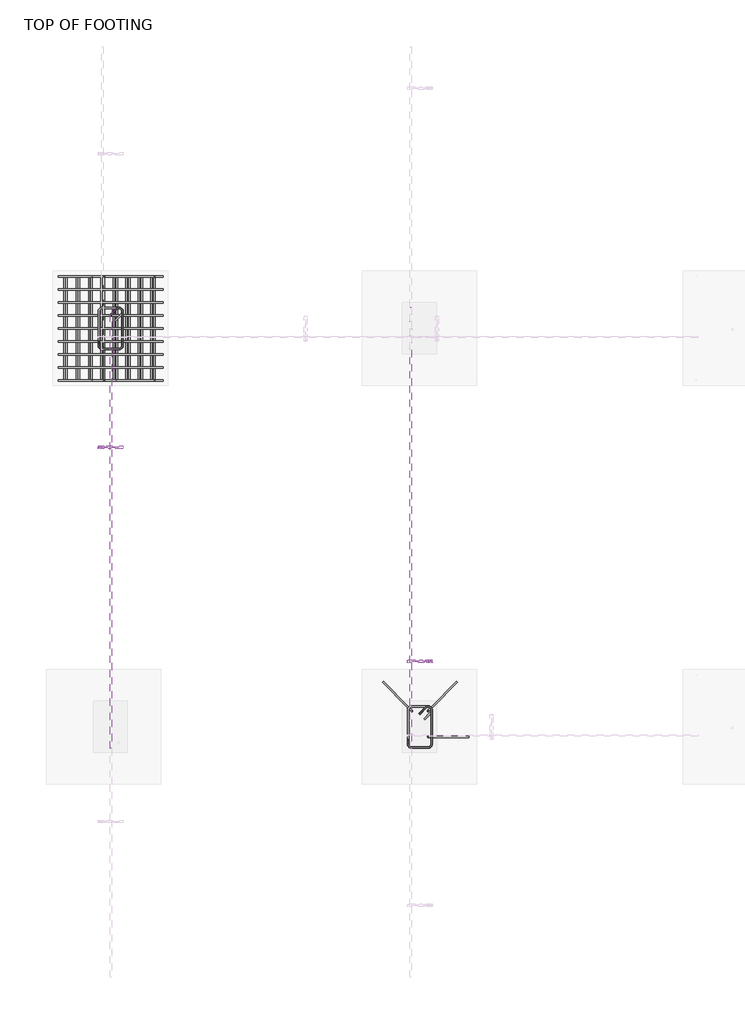
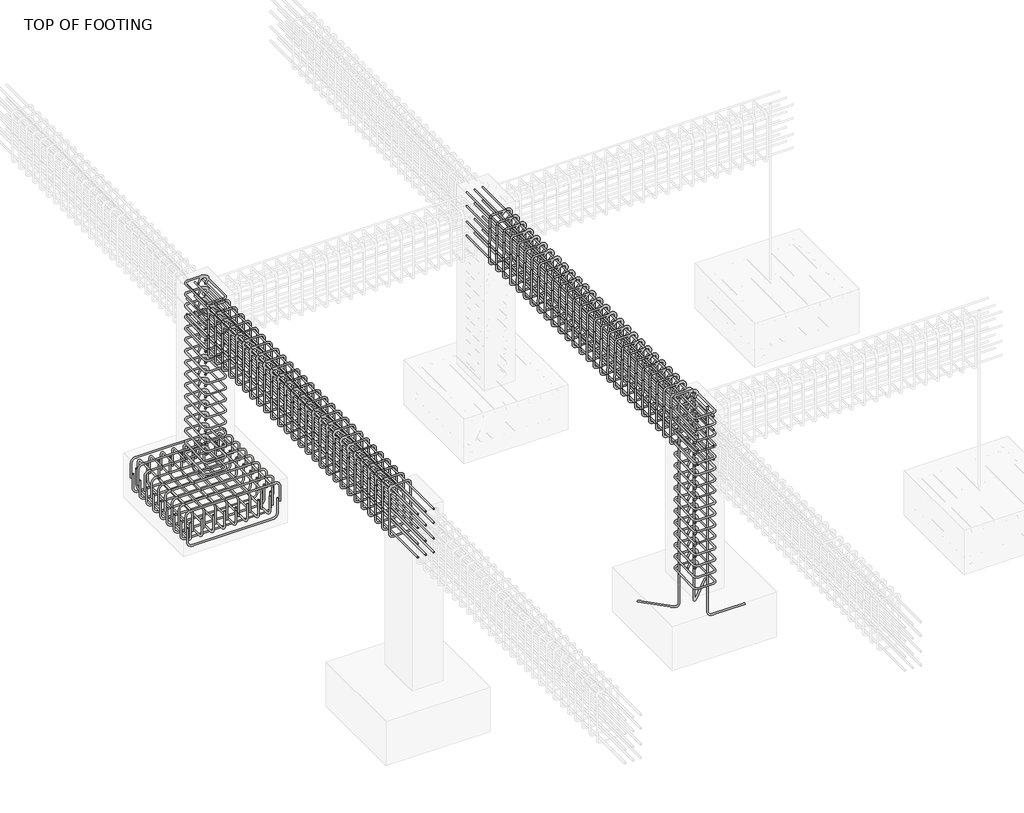
# One storey, part 6 of 14: 19 reinforcing bars.
"""IFC4 building model written with IfcOpenShell, lengths in millimetres."""

from ifc_helpers import new_model, si_unit, point, frame, origin, place, context, project, spatial, polyline, circle_curve, trimmed, segment, composite_curve, source, transform, mapped, element, save
from ifc_brep_helpers import swept_disk

model = new_model("IFC4")

# Units and contexts
model_context = context("Model", 3, world=origin())
ifc_project = project(units=[si_unit("LENGTHUNIT", "METRE", prefix="MILLI")], contexts=[model_context])

# Site, building, storey
site = spatial("IfcSite", under=ifc_project)
building = spatial("IfcBuilding", under=site)
storey = spatial("IfcBuildingStorey", under=building, Name="TOP OF FOOTING", Elevation=-1828.8)

# Reinforcing bars
placement = place(None, origin())
reinforcing_bar_shape = source(origin(), model_context, "Body", "SolidModel", [
    swept_disk(composite_curve([segment(polyline([(-3027.457813, 7055.1438575, -2035.6107622), (-3027.457813, 7055.1438575, -2182.9107622)]), True, "CONTINUOUS"), segment(trimmed(circle_curve(frame((-3073.807813, 7055.1438575, -2182.9107622), z_axis=(0.0, 1.0, 0.0), x_axis=(46.34999999999991, 0.0, 0.0)), 46.35), [point((-3027.457813, 7055.1438575, -2182.9107622))], [point((-3073.807813, 7055.1438575, -2229.2607622))], True, "CARTESIAN"), True, "CONTINUOUS"), segment(polyline([(-3073.807813, 7055.1438575, -2229.2607622), (-3846.4382016, 7055.1438575, -2229.2607622)]), True, "CONTINUOUS"), segment(trimmed(circle_curve(frame((-3846.4382016, 7055.1438575, -2182.9107622), z_axis=(0.0, 1.0, 0.0), x_axis=(0.0, 0.0, -46.34999999999991)), 46.35), [point((-3846.4382016, 7055.1438575, -2229.2607622))], [point((-3892.7882016, 7055.1438575, -2182.9107622))], True, "CARTESIAN"), True, "CONTINUOUS"), segment(polyline([(-3892.7882016, 7055.1438575, -2182.9107622), (-3892.7882016, 7055.1438575, -2035.6107622)]), True, "CONTINUOUS")], self_intersect=False), 6.35),
])
element("IfcReinforcingBar", 1, at=placement, inside=storey, context=model_context, shape_type="MappedRepresentation", body=[
    mapped(reinforcing_bar_shape, transform((0.0, 0.0, 0.0), x_axis=(1.0, 0.0, 0.0), y_axis=(0.0, 1.0, 0.0), z_axis=(0.0, 0.0, 1.0))),
    mapped(reinforcing_bar_shape, transform((0.0, -113.4125, 0.0), x_axis=(1.0, 0.0, 0.0), y_axis=(0.0, 1.0, 0.0), z_axis=(0.0, 0.0, 1.0))),
    mapped(reinforcing_bar_shape, transform((0.0, -226.825, 0.0), x_axis=(1.0, 0.0, 0.0), y_axis=(0.0, 1.0, 0.0), z_axis=(0.0, 0.0, 1.0))),
    mapped(reinforcing_bar_shape, transform((0.0, -340.2375, 0.0), x_axis=(1.0, 0.0, 0.0), y_axis=(0.0, 1.0, 0.0), z_axis=(0.0, 0.0, 1.0))),
    mapped(reinforcing_bar_shape, transform((0.0, -453.65, 0.0), x_axis=(1.0, 0.0, 0.0), y_axis=(0.0, 1.0, 0.0), z_axis=(0.0, 0.0, 1.0))),
    mapped(reinforcing_bar_shape, transform((0.0, -567.0625, 0.0), x_axis=(1.0, 0.0, 0.0), y_axis=(0.0, 1.0, 0.0), z_axis=(0.0, 0.0, 1.0))),
    mapped(reinforcing_bar_shape, transform((0.0, -680.475, 0.0), x_axis=(1.0, 0.0, 0.0), y_axis=(0.0, 1.0, 0.0), z_axis=(0.0, 0.0, 1.0))),
    mapped(reinforcing_bar_shape, transform((0.0, -793.8875, 0.0), x_axis=(1.0, 0.0, 0.0), y_axis=(0.0, 1.0, 0.0), z_axis=(0.0, 0.0, 1.0))),
    mapped(reinforcing_bar_shape, transform((0.0, -907.3, 0.0), x_axis=(1.0, 0.0, 0.0), y_axis=(0.0, 1.0, 0.0), z_axis=(0.0, 0.0, 1.0))),
])
reinforcing_bar_2_shape = source(origin(), model_context, "Body", "SolidModel", [
    swept_disk(composite_curve([segment(polyline([(-3911.0033787, 7055.1438575, -2068.991024), (-3911.0033787, 7055.1438575, -1921.691024)]), True, "CONTINUOUS"), segment(trimmed(circle_curve(frame((-3864.6533787, 7055.1438575, -1921.691024), z_axis=(0.0, 1.0, 0.0), x_axis=(-46.350000000000364, 0.0, 0.0)), 46.35), [point((-3911.0033787, 7055.1438575, -1921.691024))], [point((-3864.6533787, 7055.1438575, -1875.341024))], True, "CARTESIAN"), True, "CONTINUOUS"), segment(polyline([(-3864.6533787, 7055.1438575, -1875.341024), (-3050.0533787, 7055.1438575, -1875.341024)]), True, "CONTINUOUS"), segment(trimmed(circle_curve(frame((-3050.0533787, 7055.1438575, -1921.691024), z_axis=(0.0, 1.0, 0.0), x_axis=(0.0, 0.0, 46.34999999999991)), 46.35), [point((-3050.0533787, 7055.1438575, -1875.341024))], [point((-3003.7033787, 7055.1438575, -1921.691024))], True, "CARTESIAN"), True, "CONTINUOUS"), segment(polyline([(-3003.7033787, 7055.1438575, -1921.691024), (-3003.7033787, 7055.1438575, -2068.991024)]), True, "CONTINUOUS")], self_intersect=False), 6.35),
])
element("IfcReinforcingBar", 2, at=placement, inside=storey, context=model_context, shape_type="MappedRepresentation", body=[
    mapped(reinforcing_bar_2_shape, transform((0.0, 0.0, 0.0), x_axis=(1.0, 0.0, 0.0), y_axis=(0.0, 1.0, 0.0), z_axis=(0.0, 0.0, 1.0))),
    mapped(reinforcing_bar_2_shape, transform((0.0, -113.4125, 0.0), x_axis=(1.0, 0.0, 0.0), y_axis=(0.0, 1.0, 0.0), z_axis=(0.0, 0.0, 1.0))),
    mapped(reinforcing_bar_2_shape, transform((0.0, -226.825, 0.0), x_axis=(1.0, 0.0, 0.0), y_axis=(0.0, 1.0, 0.0), z_axis=(0.0, 0.0, 1.0))),
    mapped(reinforcing_bar_2_shape, transform((0.0, -340.2375, 0.0), x_axis=(1.0, 0.0, 0.0), y_axis=(0.0, 1.0, 0.0), z_axis=(0.0, 0.0, 1.0))),
    mapped(reinforcing_bar_2_shape, transform((0.0, -453.65, 0.0), x_axis=(1.0, 0.0, 0.0), y_axis=(0.0, 1.0, 0.0), z_axis=(0.0, 0.0, 1.0))),
    mapped(reinforcing_bar_2_shape, transform((0.0, -567.0625, 0.0), x_axis=(1.0, 0.0, 0.0), y_axis=(0.0, 1.0, 0.0), z_axis=(0.0, 0.0, 1.0))),
    mapped(reinforcing_bar_2_shape, transform((0.0, -680.475, 0.0), x_axis=(1.0, 0.0, 0.0), y_axis=(0.0, 1.0, 0.0), z_axis=(0.0, 0.0, 1.0))),
    mapped(reinforcing_bar_2_shape, transform((0.0, -793.8875, 0.0), x_axis=(1.0, 0.0, 0.0), y_axis=(0.0, 1.0, 0.0), z_axis=(0.0, 0.0, 1.0))),
    mapped(reinforcing_bar_2_shape, transform((0.0, -907.3, 0.0), x_axis=(1.0, 0.0, 0.0), y_axis=(0.0, 1.0, 0.0), z_axis=(0.0, 0.0, 1.0))),
])
reinforcing_bar_3_shape = source(origin(), model_context, "Body", "SolidModel", [
    swept_disk(composite_curve([segment(polyline([(-3073.4932847, 7055.1438575, -2085.4684936), (-3073.4932847, 7055.1438575, -1938.1684936)]), True, "CONTINUOUS"), segment(trimmed(circle_curve(frame((-3073.4932847, 7008.7938575, -1938.1684936), z_axis=(1.0, 0.0, 0.0), x_axis=(0.0, 46.350000000000364, 0.0)), 46.35), [point((-3073.4932847, 7055.1438575, -1938.1684936))], [point((-3073.4932847, 7008.7938575, -1891.8184936))], True, "CARTESIAN"), True, "CONTINUOUS"), segment(polyline([(-3073.4932847, 7008.7938575, -1891.8184936), (-3073.4932847, 6194.1938575, -1891.8184936)]), True, "CONTINUOUS"), segment(trimmed(circle_curve(frame((-3073.4932847, 6194.1938575, -1938.1684936), z_axis=(1.0, 0.0, 0.0), x_axis=(0.0, 0.0, 46.34999999999991)), 46.35), [point((-3073.4932847, 6194.1938575, -1891.8184936))], [point((-3073.4932847, 6147.8438575, -1938.1684936))], True, "CARTESIAN"), True, "CONTINUOUS"), segment(polyline([(-3073.4932847, 6147.8438575, -1938.1684936), (-3073.4932847, 6147.8438575, -2085.4684936)]), True, "CONTINUOUS")], self_intersect=False), 6.35),
])
element("IfcReinforcingBar", 3, at=placement, inside=storey, context=model_context, shape_type="MappedRepresentation", body=[
    mapped(reinforcing_bar_3_shape, transform((0.0, 0.0, 0.0), x_axis=(1.0, 0.0, 0.0), y_axis=(0.0, 1.0, 0.0), z_axis=(0.0, 0.0, 1.0))),
    mapped(reinforcing_bar_3_shape, transform((-110.0713853, 0.0, 0.0), x_axis=(1.0, 0.0, 0.0), y_axis=(0.0, 1.0, 0.0), z_axis=(0.0, 0.0, 1.0))),
    mapped(reinforcing_bar_3_shape, transform((-220.1427706, 0.0, 0.0), x_axis=(1.0, 0.0, 0.0), y_axis=(0.0, 1.0, 0.0), z_axis=(0.0, 0.0, 1.0))),
    mapped(reinforcing_bar_3_shape, transform((-330.2141558, 0.0, 0.0), x_axis=(1.0, 0.0, 0.0), y_axis=(0.0, 1.0, 0.0), z_axis=(0.0, 0.0, 1.0))),
    mapped(reinforcing_bar_3_shape, transform((-440.2855411, 0.0, 0.0), x_axis=(1.0, 0.0, 0.0), y_axis=(0.0, 1.0, 0.0), z_axis=(0.0, 0.0, 1.0))),
    mapped(reinforcing_bar_3_shape, transform((-550.3569264, 0.0, 0.0), x_axis=(1.0, 0.0, 0.0), y_axis=(0.0, 1.0, 0.0), z_axis=(0.0, 0.0, 1.0))),
    mapped(reinforcing_bar_3_shape, transform((-660.4283117, 0.0, 0.0), x_axis=(1.0, 0.0, 0.0), y_axis=(0.0, 1.0, 0.0), z_axis=(0.0, 0.0, 1.0))),
    mapped(reinforcing_bar_3_shape, transform((-770.4996969, 0.0, 0.0), x_axis=(1.0, 0.0, 0.0), y_axis=(0.0, 1.0, 0.0), z_axis=(0.0, 0.0, 1.0))),
])
reinforcing_bar_4_shape = source(origin(), model_context, "Body", "SolidModel", [
    swept_disk(composite_curve([segment(polyline([(-3862.3533787, 7055.1438575, -1990.15), (-3862.3533787, 7055.1438575, -2137.45)]), True, "CONTINUOUS"), segment(trimmed(circle_curve(frame((-3862.3533787, 7008.7938575, -2137.45), z_axis=(-1.0, 0.0, 0.0), x_axis=(0.0, 46.350000000000364, 0.0)), 46.35), [point((-3862.3533787, 7055.1438575, -2137.45))], [point((-3862.3533787, 7008.7938575, -2183.8))], True, "CARTESIAN"), True, "CONTINUOUS"), segment(polyline([(-3862.3533787, 7008.7938575, -2183.8), (-3862.3533787, 6194.1938575, -2183.8)]), True, "CONTINUOUS"), segment(trimmed(circle_curve(frame((-3862.3533787, 6194.1938575, -2137.45), z_axis=(-1.0, 0.0, 0.0), x_axis=(0.0, 0.0, -46.350000000000364)), 46.35), [point((-3862.3533787, 6194.1938575, -2183.8))], [point((-3862.3533787, 6147.8438575, -2137.45))], True, "CARTESIAN"), True, "CONTINUOUS"), segment(polyline([(-3862.3533787, 6147.8438575, -2137.45), (-3862.3533787, 6147.8438575, -1990.15)]), True, "CONTINUOUS")], self_intersect=False), 6.35),
])
element("IfcReinforcingBar", 4, at=placement, inside=storey, context=model_context, shape_type="MappedRepresentation", body=[
    mapped(reinforcing_bar_4_shape, transform((0.0, 0.0, 0.0), x_axis=(1.0, 0.0, 0.0), y_axis=(0.0, 1.0, 0.0), z_axis=(0.0, 0.0, 1.0))),
    mapped(reinforcing_bar_4_shape, transform((108.7810905, 0.0, 0.0), x_axis=(1.0, 0.0, 0.0), y_axis=(0.0, 1.0, 0.0), z_axis=(0.0, 0.0, 1.0))),
    mapped(reinforcing_bar_4_shape, transform((217.5621811, 0.0, 0.0), x_axis=(1.0, 0.0, 0.0), y_axis=(0.0, 1.0, 0.0), z_axis=(0.0, 0.0, 1.0))),
    mapped(reinforcing_bar_4_shape, transform((326.3432716, 0.0, 0.0), x_axis=(1.0, 0.0, 0.0), y_axis=(0.0, 1.0, 0.0), z_axis=(0.0, 0.0, 1.0))),
    mapped(reinforcing_bar_4_shape, transform((435.1243621, 0.0, 0.0), x_axis=(1.0, 0.0, 0.0), y_axis=(0.0, 1.0, 0.0), z_axis=(0.0, 0.0, 1.0))),
    mapped(reinforcing_bar_4_shape, transform((543.9054526, 0.0, 0.0), x_axis=(1.0, 0.0, 0.0), y_axis=(0.0, 1.0, 0.0), z_axis=(0.0, 0.0, 1.0))),
    mapped(reinforcing_bar_4_shape, transform((652.6865432, 0.0, 0.0), x_axis=(1.0, 0.0, 0.0), y_axis=(0.0, 1.0, 0.0), z_axis=(0.0, 0.0, 1.0))),
    mapped(reinforcing_bar_4_shape, transform((761.4676337, 0.0, 0.0), x_axis=(1.0, 0.0, 0.0), y_axis=(0.0, 1.0, 0.0), z_axis=(0.0, 0.0, 1.0))),
])
reinforcing_bar_5_shape = source(origin(), model_context, "Body", "SolidModel", [
    swept_disk(composite_curve([segment(polyline([(-3462.9647392, 6715.2180921, -46.35), (-3407.2211763, 6770.9616551, -46.35)]), True, "CONTINUOUS"), segment(trimmed(circle_curve(frame((-3385.0533787, 6748.7938575, -46.35), z_axis=(0.0, 0.0, -1.0), x_axis=(-22.167797600000085, 22.167797600000085, 0.0)), 31.35), [point((-3407.2211763, 6770.9616551, -46.35))], [point((-3353.7033787, 6748.7938575, -46.35))], True, "CARTESIAN"), True, "CONTINUOUS"), segment(polyline([(-3353.7033787, 6748.7938575, -46.35), (-3353.7033787, 6454.1938575, -46.35)]), True, "CONTINUOUS"), segment(trimmed(circle_curve(frame((-3385.0533787, 6454.1938575, -46.35), z_axis=(0.0, 0.0, -1.0), x_axis=(31.34999999999991, 0.0, 0.0)), 31.35), [point((-3353.7033787, 6454.1938575, -46.35))], [point((-3385.0533787, 6422.8438575, -46.35))], True, "CARTESIAN"), True, "CONTINUOUS"), segment(polyline([(-3385.0533787, 6422.8438575, -46.35), (-3529.6533787, 6422.8438575, -46.35)]), True, "CONTINUOUS"), segment(trimmed(circle_curve(frame((-3529.6533787, 6454.1740724, -45.2363875), z_axis=(0.0, 0.03552192833448213, -0.9993688971583016), x_axis=(0.0, -31.3302149000001, -1.1136125000000021)), 31.35), [point((-3529.6533787, 6422.8438575, -46.35))], [point((-3561.0033787, 6454.1740724, -45.2363875))], True, "CARTESIAN"), True, "CONTINUOUS"), segment(polyline([(-3561.0033787, 6454.1740724, -45.2363875), (-3561.0033787, 6748.8136426, -34.7636125)]), True, "CONTINUOUS"), segment(trimmed(circle_curve(frame((-3529.6533787, 6748.8136426, -34.7636125), z_axis=(0.0, 0.03552192833448213, -0.9993688971583016), x_axis=(-31.350000000000364, 0.0, 0.0)), 31.35), [point((-3561.0033787, 6748.8136426, -34.7636125))], [point((-3529.6533787, 6780.1438575, -33.65))], True, "CARTESIAN"), True, "CONTINUOUS"), segment(polyline([(-3529.6533787, 6780.1438575, -33.65), (-3385.0533787, 6780.1438575, -33.65)]), True, "CONTINUOUS"), segment(trimmed(circle_curve(frame((-3385.0533787, 6748.7938575, -33.65), z_axis=(0.0, 0.0, -1.0), x_axis=(0.0, 31.350000000000364, 0.0)), 31.35), [point((-3385.0533787, 6780.1438575, -33.65))], [point((-3362.8855811, 6726.6260599, -33.65))], True, "CARTESIAN"), True, "CONTINUOUS"), segment(polyline([(-3362.8855811, 6726.6260599, -33.65), (-3418.6291441, 6670.8824969, -33.65)]), True, "CONTINUOUS")], self_intersect=False), 6.35),
])
element("IfcReinforcingBar", 5, at=placement, inside=storey, context=model_context, shape_type="MappedRepresentation", body=[
    mapped(reinforcing_bar_5_shape, transform((0.0, 0.0, 0.0), x_axis=(1.0, 0.0, 0.0), y_axis=(0.0, 1.0, 0.0), z_axis=(0.0, 0.0, 1.0))),
    mapped(reinforcing_bar_5_shape, transform((0.0, 0.0, -115.74), x_axis=(1.0, 0.0, 0.0), y_axis=(0.0, 1.0, 0.0), z_axis=(0.0, 0.0, 1.0))),
    mapped(reinforcing_bar_5_shape, transform((0.0, 0.0, -231.48), x_axis=(1.0, 0.0, 0.0), y_axis=(0.0, 1.0, 0.0), z_axis=(0.0, 0.0, 1.0))),
    mapped(reinforcing_bar_5_shape, transform((0.0, 0.0, -347.22), x_axis=(1.0, 0.0, 0.0), y_axis=(0.0, 1.0, 0.0), z_axis=(0.0, 0.0, 1.0))),
    mapped(reinforcing_bar_5_shape, transform((0.0, 0.0, -462.96), x_axis=(1.0, 0.0, 0.0), y_axis=(0.0, 1.0, 0.0), z_axis=(0.0, 0.0, 1.0))),
    mapped(reinforcing_bar_5_shape, transform((0.0, 0.0, -578.7), x_axis=(1.0, 0.0, 0.0), y_axis=(0.0, 1.0, 0.0), z_axis=(0.0, 0.0, 1.0))),
    mapped(reinforcing_bar_5_shape, transform((0.0, 0.0, -694.44), x_axis=(1.0, 0.0, 0.0), y_axis=(0.0, 1.0, 0.0), z_axis=(0.0, 0.0, 1.0))),
    mapped(reinforcing_bar_5_shape, transform((0.0, 0.0, -810.18), x_axis=(1.0, 0.0, 0.0), y_axis=(0.0, 1.0, 0.0), z_axis=(0.0, 0.0, 1.0))),
    mapped(reinforcing_bar_5_shape, transform((0.0, 0.0, -925.92), x_axis=(1.0, 0.0, 0.0), y_axis=(0.0, 1.0, 0.0), z_axis=(0.0, 0.0, 1.0))),
    mapped(reinforcing_bar_5_shape, transform((0.0, 0.0, -1041.66), x_axis=(1.0, 0.0, 0.0), y_axis=(0.0, 1.0, 0.0), z_axis=(0.0, 0.0, 1.0))),
    mapped(reinforcing_bar_5_shape, transform((0.0, 0.0, -1157.4), x_axis=(1.0, 0.0, 0.0), y_axis=(0.0, 1.0, 0.0), z_axis=(0.0, 0.0, 1.0))),
    mapped(reinforcing_bar_5_shape, transform((0.0, 0.0, -1273.14), x_axis=(1.0, 0.0, 0.0), y_axis=(0.0, 1.0, 0.0), z_axis=(0.0, 0.0, 1.0))),
    mapped(reinforcing_bar_5_shape, transform((0.0, 0.0, -1388.88), x_axis=(1.0, 0.0, 0.0), y_axis=(0.0, 1.0, 0.0), z_axis=(0.0, 0.0, 1.0))),
    mapped(reinforcing_bar_5_shape, transform((0.0, 0.0, -1504.62), x_axis=(1.0, 0.0, 0.0), y_axis=(0.0, 1.0, 0.0), z_axis=(0.0, 0.0, 1.0))),
    mapped(reinforcing_bar_5_shape, transform((0.0, 0.0, -1620.36), x_axis=(1.0, 0.0, 0.0), y_axis=(0.0, 1.0, 0.0), z_axis=(0.0, 0.0, 1.0))),
    mapped(reinforcing_bar_5_shape, transform((0.0, 0.0, -1736.1), x_axis=(1.0, 0.0, 0.0), y_axis=(0.0, 1.0, 0.0), z_axis=(0.0, 0.0, 1.0))),
])
reinforcing_bar_6_shape = source(origin(), model_context, "Body", "SolidModel", [
    swept_disk(composite_curve([segment(polyline([(-762.9647392, 3237.9741144, -46.35), (-707.2211763, 3293.7176774, -46.35)]), True, "CONTINUOUS"), segment(trimmed(circle_curve(frame((-685.0533787, 3271.5498798, -46.35), z_axis=(0.0, 0.0, -1.0), x_axis=(-22.16779759999997, 22.167797600000085, 0.0)), 31.35), [point((-707.2211763, 3293.7176774, -46.35))], [point((-653.7033787, 3271.5498798, -46.35))], True, "CARTESIAN"), True, "CONTINUOUS"), segment(polyline([(-653.7033787, 3271.5498798, -46.35), (-653.7033787, 2976.9498798, -46.35)]), True, "CONTINUOUS"), segment(trimmed(circle_curve(frame((-685.0533787, 2976.9498798, -46.35), z_axis=(0.0, 0.0, -1.0), x_axis=(31.350000000000023, 0.0, 0.0)), 31.35), [point((-653.7033787, 2976.9498798, -46.35))], [point((-685.0533787, 2945.5998798, -46.35))], True, "CARTESIAN"), True, "CONTINUOUS"), segment(polyline([(-685.0533787, 2945.5998798, -46.35), (-829.6533787, 2945.5998798, -46.35)]), True, "CONTINUOUS"), segment(trimmed(circle_curve(frame((-829.6533787, 2976.9300947, -45.2363875), z_axis=(0.0, 0.03552192833448213, -0.9993688971583016), x_axis=(0.0, -31.3302149000001, -1.1136125000000021)), 31.35), [point((-829.6533787, 2945.5998798, -46.35))], [point((-861.0033787, 2976.9300947, -45.2363875))], True, "CARTESIAN"), True, "CONTINUOUS"), segment(polyline([(-861.0033787, 2976.9300947, -45.2363875), (-861.0033787, 3271.5696648, -34.7636125)]), True, "CONTINUOUS"), segment(trimmed(circle_curve(frame((-829.6533787, 3271.5696648, -34.7636125), z_axis=(0.0, 0.03552192833448213, -0.9993688971583016), x_axis=(-31.350000000000023, 0.0, 0.0)), 31.35), [point((-861.0033787, 3271.5696648, -34.7636125))], [point((-829.6533787, 3302.8998798, -33.65))], True, "CARTESIAN"), True, "CONTINUOUS"), segment(polyline([(-829.6533787, 3302.8998798, -33.65), (-685.0533787, 3302.8998798, -33.65)]), True, "CONTINUOUS"), segment(trimmed(circle_curve(frame((-685.0533787, 3271.5498798, -33.65), z_axis=(0.0, 0.0, -1.0), x_axis=(0.0, 31.34999999999991, 0.0)), 31.35), [point((-685.0533787, 3302.8998798, -33.65))], [point((-662.8855811, 3249.3820822, -33.65))], True, "CARTESIAN"), True, "CONTINUOUS"), segment(polyline([(-662.8855811, 3249.3820822, -33.65), (-718.6291441, 3193.6385192, -33.65)]), True, "CONTINUOUS")], self_intersect=False), 6.35),
])
element("IfcReinforcingBar", 6, at=placement, inside=storey, context=model_context, shape_type="MappedRepresentation", body=[
    mapped(reinforcing_bar_6_shape, transform((0.0, 0.0, 0.0), x_axis=(1.0, 0.0, 0.0), y_axis=(0.0, 1.0, 0.0), z_axis=(0.0, 0.0, 1.0))),
    mapped(reinforcing_bar_6_shape, transform((0.0, 0.0, -115.74), x_axis=(1.0, 0.0, 0.0), y_axis=(0.0, 1.0, 0.0), z_axis=(0.0, 0.0, 1.0))),
    mapped(reinforcing_bar_6_shape, transform((0.0, 0.0, -231.48), x_axis=(1.0, 0.0, 0.0), y_axis=(0.0, 1.0, 0.0), z_axis=(0.0, 0.0, 1.0))),
    mapped(reinforcing_bar_6_shape, transform((0.0, 0.0, -347.22), x_axis=(1.0, 0.0, 0.0), y_axis=(0.0, 1.0, 0.0), z_axis=(0.0, 0.0, 1.0))),
    mapped(reinforcing_bar_6_shape, transform((0.0, 0.0, -462.96), x_axis=(1.0, 0.0, 0.0), y_axis=(0.0, 1.0, 0.0), z_axis=(0.0, 0.0, 1.0))),
    mapped(reinforcing_bar_6_shape, transform((0.0, 0.0, -578.7), x_axis=(1.0, 0.0, 0.0), y_axis=(0.0, 1.0, 0.0), z_axis=(0.0, 0.0, 1.0))),
    mapped(reinforcing_bar_6_shape, transform((0.0, 0.0, -694.44), x_axis=(1.0, 0.0, 0.0), y_axis=(0.0, 1.0, 0.0), z_axis=(0.0, 0.0, 1.0))),
    mapped(reinforcing_bar_6_shape, transform((0.0, 0.0, -810.18), x_axis=(1.0, 0.0, 0.0), y_axis=(0.0, 1.0, 0.0), z_axis=(0.0, 0.0, 1.0))),
    mapped(reinforcing_bar_6_shape, transform((0.0, 0.0, -925.92), x_axis=(1.0, 0.0, 0.0), y_axis=(0.0, 1.0, 0.0), z_axis=(0.0, 0.0, 1.0))),
    mapped(reinforcing_bar_6_shape, transform((0.0, 0.0, -1041.66), x_axis=(1.0, 0.0, 0.0), y_axis=(0.0, 1.0, 0.0), z_axis=(0.0, 0.0, 1.0))),
    mapped(reinforcing_bar_6_shape, transform((0.0, 0.0, -1157.4), x_axis=(1.0, 0.0, 0.0), y_axis=(0.0, 1.0, 0.0), z_axis=(0.0, 0.0, 1.0))),
    mapped(reinforcing_bar_6_shape, transform((0.0, 0.0, -1273.14), x_axis=(1.0, 0.0, 0.0), y_axis=(0.0, 1.0, 0.0), z_axis=(0.0, 0.0, 1.0))),
    mapped(reinforcing_bar_6_shape, transform((0.0, 0.0, -1388.88), x_axis=(1.0, 0.0, 0.0), y_axis=(0.0, 1.0, 0.0), z_axis=(0.0, 0.0, 1.0))),
    mapped(reinforcing_bar_6_shape, transform((0.0, 0.0, -1504.62), x_axis=(1.0, 0.0, 0.0), y_axis=(0.0, 1.0, 0.0), z_axis=(0.0, 0.0, 1.0))),
    mapped(reinforcing_bar_6_shape, transform((0.0, 0.0, -1620.36), x_axis=(1.0, 0.0, 0.0), y_axis=(0.0, 1.0, 0.0), z_axis=(0.0, 0.0, 1.0))),
    mapped(reinforcing_bar_6_shape, transform((0.0, 0.0, -1736.1), x_axis=(1.0, 0.0, 0.0), y_axis=(0.0, 1.0, 0.0), z_axis=(0.0, 0.0, 1.0))),
])
element("IfcReinforcingBar", 7, at=placement, inside=storey, context=model_context, shape_type="SolidModel", body=[
    swept_disk(composite_curve([segment(polyline([(-686.7020371, 3039.1707812, -40.0), (-686.7020371, 3039.1707812, -2122.4113862)]), True, "CONTINUOUS"), segment(trimmed(circle_curve(frame((-640.3520371, 3039.1707812, -2122.4113862), z_axis=(0.0, -1.0, 0.0), x_axis=(-46.35000000000002, 0.0, 0.0)), 46.35), [point((-686.7020371, 3039.1707812, -2122.4113862))], [point((-640.3520371, 3039.1707812, -2168.7613862))], True, "CARTESIAN"), True, "CONTINUOUS"), segment(polyline([(-640.3520371, 3039.1707812, -2168.7613862), (-328.2406023, 3039.1707812, -2168.7613862)]), True, "CONTINUOUS")], self_intersect=False), 6.35),
])
element("IfcReinforcingBar", 8, at=placement, inside=storey, context=model_context, shape_type="SolidModel", body=[
    swept_disk(composite_curve([segment(polyline([(-686.7020371, 3264.3289783, -40.0), (-686.7020371, 3264.3289783, -2122.4113862)]), True, "CONTINUOUS"), segment(trimmed(circle_curve(frame((-653.9276378, 3297.1033776, -2122.4113862), z_axis=(0.7071067811865235, -0.7071067811865717, 0.0), x_axis=(-32.77439930000003, -32.774399299999914, 0.0)), 46.35), [point((-686.7020371, 3264.3289783, -2122.4113862))], [point((-653.9276378, 3297.1033776, -2168.7613862))], True, "CARTESIAN"), True, "CONTINUOUS"), segment(polyline([(-653.9276378, 3297.1033776, -2168.7613862), (-433.2315258, 3517.7994896, -2168.7613862)]), True, "CONTINUOUS")], self_intersect=False), 6.35),
])
element("IfcReinforcingBar", 9, at=placement, inside=storey, context=model_context, shape_type="SolidModel", body=[
    swept_disk(composite_curve([segment(polyline([(-828.0047203, 3264.3289783, -40.0), (-828.0047203, 3264.3289783, -2122.4113862)]), True, "CONTINUOUS"), segment(trimmed(circle_curve(frame((-860.7791196, 3297.1033776, -2122.4113862), z_axis=(0.7071067811865548, 0.7071067811865404, 0.0), x_axis=(32.774399299999914, -32.774399299999914, 0.0)), 46.35), [point((-828.0047203, 3264.3289783, -2122.4113862))], [point((-860.7791196, 3297.1033776, -2168.7613862))], True, "CARTESIAN"), True, "CONTINUOUS"), segment(polyline([(-860.7791196, 3297.1033776, -2168.7613862), (-1081.4752316, 3517.7994896, -2168.7613862)]), True, "CONTINUOUS")], self_intersect=False), 6.35),
])
reinforcing_bar_7_shape = source(origin(), model_context, "Body", "SolidModel", [
    swept_disk(composite_curve([segment(polyline([(-3451.7420182, 6370.1438575, -111.2757654), (-3507.4855811, 6370.1438575, -55.5322024)]), True, "CONTINUOUS"), segment(trimmed(circle_curve(frame((-3529.6533787, 6370.1438575, -77.7), z_axis=(0.0, -1.0, 0.0), x_axis=(22.16779759999963, 0.0, 22.1677976)), 31.35), [point((-3507.4855811, 6370.1438575, -55.5322024))], [point((-3561.0033787, 6370.1438575, -77.7))], True, "CARTESIAN"), True, "CONTINUOUS"), segment(polyline([(-3561.0033787, 6370.1438575, -77.7), (-3561.0033787, 6370.1438575, -522.3)]), True, "CONTINUOUS"), segment(trimmed(circle_curve(frame((-3529.6533787, 6370.1438575, -522.3), z_axis=(0.0, -1.0, 0.0), x_axis=(-31.350000000000364, 0.0, 0.0)), 31.35), [point((-3561.0033787, 6370.1438575, -522.3))], [point((-3529.6533787, 6370.1438575, -553.65))], True, "CARTESIAN"), True, "CONTINUOUS"), segment(polyline([(-3529.6533787, 6370.1438575, -553.65), (-3385.0533787, 6370.1438575, -553.65)]), True, "CONTINUOUS"), segment(trimmed(circle_curve(frame((-3385.0533787, 6370.9284431, -522.3098193), z_axis=(0.0, -0.9996867842138424, 0.025026655153786322), x_axis=(0.0, -0.7845855999994455, -31.34018070000002)), 31.35), [point((-3385.0533787, 6370.1438575, -553.65))], [point((-3353.7033787, 6370.9284431, -522.3098193))], True, "CARTESIAN"), True, "CONTINUOUS"), segment(polyline([(-3353.7033787, 6370.9284431, -522.3098193), (-3353.7033787, 6382.0592718, -77.6901807)]), True, "CONTINUOUS"), segment(trimmed(circle_curve(frame((-3385.0533787, 6382.0592718, -77.6901807), z_axis=(0.0, -0.9996867842138424, 0.025026655153786322), x_axis=(31.34999999999991, 0.0, 0.0)), 31.35), [point((-3353.7033787, 6382.0592718, -77.6901807))], [point((-3385.0533787, 6382.8438575, -46.35))], True, "CARTESIAN"), True, "CONTINUOUS"), segment(polyline([(-3385.0533787, 6382.8438575, -46.35), (-3529.6533787, 6382.8438575, -46.35)]), True, "CONTINUOUS"), segment(trimmed(circle_curve(frame((-3529.6533787, 6382.8438575, -77.7), z_axis=(0.0, -1.0, 0.0), x_axis=(0.0, 0.0, 31.35)), 31.35), [point((-3529.6533787, 6382.8438575, -46.35))], [point((-3551.8211763, 6382.8438575, -99.8677976))], True, "CARTESIAN"), True, "CONTINUOUS"), segment(polyline([(-3551.8211763, 6382.8438575, -99.8677976), (-3496.0776133, 6382.8438575, -155.6113605)]), True, "CONTINUOUS")], self_intersect=False), 6.35),
])
element("IfcReinforcingBar", 10, at=placement, inside=storey, context=model_context, shape_type="MappedRepresentation", body=[
    mapped(reinforcing_bar_7_shape, transform((0.0, 0.0, 0.0), x_axis=(1.0, 0.0, 0.0), y_axis=(0.0, 1.0, 0.0), z_axis=(0.0, 0.0, 1.0))),
    mapped(reinforcing_bar_7_shape, transform((0.0, -115.9439991, 0.0), x_axis=(1.0, 0.0, 0.0), y_axis=(0.0, 1.0, 0.0), z_axis=(0.0, 0.0, 1.0))),
    mapped(reinforcing_bar_7_shape, transform((0.0, -231.8879983, 0.0), x_axis=(1.0, 0.0, 0.0), y_axis=(0.0, 1.0, 0.0), z_axis=(0.0, 0.0, 1.0))),
    mapped(reinforcing_bar_7_shape, transform((0.0, -347.8319974, 0.0), x_axis=(1.0, 0.0, 0.0), y_axis=(0.0, 1.0, 0.0), z_axis=(0.0, 0.0, 1.0))),
    mapped(reinforcing_bar_7_shape, transform((0.0, -463.7759966, 0.0), x_axis=(1.0, 0.0, 0.0), y_axis=(0.0, 1.0, 0.0), z_axis=(0.0, 0.0, 1.0))),
    mapped(reinforcing_bar_7_shape, transform((0.0, -579.7199957, 0.0), x_axis=(1.0, 0.0, 0.0), y_axis=(0.0, 1.0, 0.0), z_axis=(0.0, 0.0, 1.0))),
    mapped(reinforcing_bar_7_shape, transform((0.0, -695.6639949, 0.0), x_axis=(1.0, 0.0, 0.0), y_axis=(0.0, 1.0, 0.0), z_axis=(0.0, 0.0, 1.0))),
    mapped(reinforcing_bar_7_shape, transform((0.0, -811.607994, 0.0), x_axis=(1.0, 0.0, 0.0), y_axis=(0.0, 1.0, 0.0), z_axis=(0.0, 0.0, 1.0))),
    mapped(reinforcing_bar_7_shape, transform((0.0, -927.5519931, 0.0), x_axis=(1.0, 0.0, 0.0), y_axis=(0.0, 1.0, 0.0), z_axis=(0.0, 0.0, 1.0))),
    mapped(reinforcing_bar_7_shape, transform((0.0, -1043.4959923, 0.0), x_axis=(1.0, 0.0, 0.0), y_axis=(0.0, 1.0, 0.0), z_axis=(0.0, 0.0, 1.0))),
    mapped(reinforcing_bar_7_shape, transform((0.0, -1159.4399914, 0.0), x_axis=(1.0, 0.0, 0.0), y_axis=(0.0, 1.0, 0.0), z_axis=(0.0, 0.0, 1.0))),
    mapped(reinforcing_bar_7_shape, transform((0.0, -1275.3839906, 0.0), x_axis=(1.0, 0.0, 0.0), y_axis=(0.0, 1.0, 0.0), z_axis=(0.0, 0.0, 1.0))),
    mapped(reinforcing_bar_7_shape, transform((0.0, -1391.3279897, 0.0), x_axis=(1.0, 0.0, 0.0), y_axis=(0.0, 1.0, 0.0), z_axis=(0.0, 0.0, 1.0))),
    mapped(reinforcing_bar_7_shape, transform((0.0, -1507.2719889, 0.0), x_axis=(1.0, 0.0, 0.0), y_axis=(0.0, 1.0, 0.0), z_axis=(0.0, 0.0, 1.0))),
    mapped(reinforcing_bar_7_shape, transform((0.0, -1623.215988, 0.0), x_axis=(1.0, 0.0, 0.0), y_axis=(0.0, 1.0, 0.0), z_axis=(0.0, 0.0, 1.0))),
    mapped(reinforcing_bar_7_shape, transform((0.0, -1739.1599871, 0.0), x_axis=(1.0, 0.0, 0.0), y_axis=(0.0, 1.0, 0.0), z_axis=(0.0, 0.0, 1.0))),
    mapped(reinforcing_bar_7_shape, transform((0.0, -1855.1039863, 0.0), x_axis=(1.0, 0.0, 0.0), y_axis=(0.0, 1.0, 0.0), z_axis=(0.0, 0.0, 1.0))),
    mapped(reinforcing_bar_7_shape, transform((0.0, -1971.0479854, 0.0), x_axis=(1.0, 0.0, 0.0), y_axis=(0.0, 1.0, 0.0), z_axis=(0.0, 0.0, 1.0))),
    mapped(reinforcing_bar_7_shape, transform((0.0, -2086.9919846, 0.0), x_axis=(1.0, 0.0, 0.0), y_axis=(0.0, 1.0, 0.0), z_axis=(0.0, 0.0, 1.0))),
    mapped(reinforcing_bar_7_shape, transform((0.0, -2202.9359837, 0.0), x_axis=(1.0, 0.0, 0.0), y_axis=(0.0, 1.0, 0.0), z_axis=(0.0, 0.0, 1.0))),
    mapped(reinforcing_bar_7_shape, transform((0.0, -2318.8799829, 0.0), x_axis=(1.0, 0.0, 0.0), y_axis=(0.0, 1.0, 0.0), z_axis=(0.0, 0.0, 1.0))),
    mapped(reinforcing_bar_7_shape, transform((0.0, -2434.823982, 0.0), x_axis=(1.0, 0.0, 0.0), y_axis=(0.0, 1.0, 0.0), z_axis=(0.0, 0.0, 1.0))),
    mapped(reinforcing_bar_7_shape, transform((0.0, -2550.7679811, 0.0), x_axis=(1.0, 0.0, 0.0), y_axis=(0.0, 1.0, 0.0), z_axis=(0.0, 0.0, 1.0))),
    mapped(reinforcing_bar_7_shape, transform((0.0, -2666.7119803, 0.0), x_axis=(1.0, 0.0, 0.0), y_axis=(0.0, 1.0, 0.0), z_axis=(0.0, 0.0, 1.0))),
    mapped(reinforcing_bar_7_shape, transform((0.0, -2782.6559794, 0.0), x_axis=(1.0, 0.0, 0.0), y_axis=(0.0, 1.0, 0.0), z_axis=(0.0, 0.0, 1.0))),
    mapped(reinforcing_bar_7_shape, transform((0.0, -2898.5999786, 0.0), x_axis=(1.0, 0.0, 0.0), y_axis=(0.0, 1.0, 0.0), z_axis=(0.0, 0.0, 1.0))),
    mapped(reinforcing_bar_7_shape, transform((0.0, -3014.5439777, 0.0), x_axis=(1.0, 0.0, 0.0), y_axis=(0.0, 1.0, 0.0), z_axis=(0.0, 0.0, 1.0))),
])
reinforcing_bar_8_shape = source(origin(), model_context, "Body", "SolidModel", [
    swept_disk(composite_curve([segment(polyline([(-3377.6071253, 6786.4938575, -77.7), (-3377.6071253, 2939.2498798, -77.7)]), True, "CONTINUOUS")], self_intersect=False), 6.35),
])
element("IfcReinforcingBar", 11, at=placement, inside=storey, context=model_context, shape_type="MappedRepresentation", body=[
    mapped(reinforcing_bar_8_shape, transform((0.0, 0.0, 0.0), x_axis=(1.0, 0.0, 0.0), y_axis=(0.0, 1.0, 0.0), z_axis=(0.0, 0.0, 1.0))),
    mapped(reinforcing_bar_8_shape, transform((-76.0102945, 0.0, 0.0), x_axis=(1.0, 0.0, 0.0), y_axis=(0.0, 1.0, 0.0), z_axis=(0.0, 0.0, 1.0))),
    mapped(reinforcing_bar_8_shape, transform((-152.0205889, 0.0, 0.0), x_axis=(1.0, 0.0, 0.0), y_axis=(0.0, 1.0, 0.0), z_axis=(0.0, 0.0, 1.0))),
])
reinforcing_bar_9_shape = source(origin(), model_context, "Body", "SolidModel", [
    swept_disk(composite_curve([segment(polyline([(-3377.6071253, 6786.4938575, -517.7), (-3377.6071253, 2939.2498798, -517.7)]), True, "CONTINUOUS")], self_intersect=False), 6.35),
])
element("IfcReinforcingBar", 12, at=placement, inside=storey, context=model_context, shape_type="MappedRepresentation", body=[
    mapped(reinforcing_bar_9_shape, transform((0.0, 0.0, 0.0), x_axis=(1.0, 0.0, 0.0), y_axis=(0.0, 1.0, 0.0), z_axis=(0.0, 0.0, 1.0))),
    mapped(reinforcing_bar_9_shape, transform((-76.0102945, 0.0, 0.0), x_axis=(1.0, 0.0, 0.0), y_axis=(0.0, 1.0, 0.0), z_axis=(0.0, 0.0, 1.0))),
    mapped(reinforcing_bar_9_shape, transform((-152.0205889, 0.0, 0.0), x_axis=(1.0, 0.0, 0.0), y_axis=(0.0, 1.0, 0.0), z_axis=(0.0, 0.0, 1.0))),
])
reinforcing_bar_10_shape = source(origin(), model_context, "Body", "SolidModel", [
    swept_disk(composite_curve([segment(polyline([(-3377.6071253, 6786.4938575, -377.7), (-3377.6071253, 2939.2498798, -377.7)]), True, "CONTINUOUS")], self_intersect=False), 6.35),
])
element("IfcReinforcingBar", 13, at=placement, inside=storey, context=model_context, shape_type="MappedRepresentation", body=[
    mapped(reinforcing_bar_10_shape, transform((0.0, 0.0, 0.0), x_axis=(1.0, 0.0, 0.0), y_axis=(0.0, 1.0, 0.0), z_axis=(0.0, 0.0, 1.0))),
    mapped(reinforcing_bar_10_shape, transform((-76.0102945, 0.0, 0.0), x_axis=(1.0, 0.0, 0.0), y_axis=(0.0, 1.0, 0.0), z_axis=(0.0, 0.0, 1.0))),
    mapped(reinforcing_bar_10_shape, transform((-152.0205889, 0.0, 0.0), x_axis=(1.0, 0.0, 0.0), y_axis=(0.0, 1.0, 0.0), z_axis=(0.0, 0.0, 1.0))),
])
reinforcing_bar_11_shape = source(origin(), model_context, "Body", "SolidModel", [
    swept_disk(composite_curve([segment(polyline([(-3377.6071253, 6786.4938575, -217.7), (-3377.6071253, 2939.2498798, -217.7)]), True, "CONTINUOUS")], self_intersect=False), 6.35),
])
element("IfcReinforcingBar", 14, at=placement, inside=storey, context=model_context, shape_type="MappedRepresentation", body=[
    mapped(reinforcing_bar_11_shape, transform((0.0, 0.0, 0.0), x_axis=(1.0, 0.0, 0.0), y_axis=(0.0, 1.0, 0.0), z_axis=(0.0, 0.0, 1.0))),
    mapped(reinforcing_bar_11_shape, transform((-76.0102945, 0.0, 0.0), x_axis=(1.0, 0.0, 0.0), y_axis=(0.0, 1.0, 0.0), z_axis=(0.0, 0.0, 1.0))),
    mapped(reinforcing_bar_11_shape, transform((-152.0205889, 0.0, 0.0), x_axis=(1.0, 0.0, 0.0), y_axis=(0.0, 1.0, 0.0), z_axis=(0.0, 0.0, 1.0))),
])
reinforcing_bar_12_shape = source(origin(), model_context, "Body", "SolidModel", [
    swept_disk(composite_curve([segment(polyline([(-762.9647392, 3355.5998798, -111.2757654), (-707.2211763, 3355.5998798, -55.5322024)]), True, "CONTINUOUS"), segment(trimmed(circle_curve(frame((-685.0533787, 3355.5998798, -77.7), z_axis=(0.0, 1.0, 0.0), x_axis=(-22.16779759999997, 0.0, 22.1677976)), 31.35), [point((-707.2211763, 3355.5998798, -55.5322024))], [point((-653.7033787, 3355.5998798, -77.7))], True, "CARTESIAN"), True, "CONTINUOUS"), segment(polyline([(-653.7033787, 3355.5998798, -77.7), (-653.7033787, 3355.5998798, -522.3)]), True, "CONTINUOUS"), segment(trimmed(circle_curve(frame((-685.0533787, 3355.5998798, -522.3), z_axis=(0.0, 1.0, 0.0), x_axis=(31.350000000000023, 0.0, 0.0)), 31.35), [point((-653.7033787, 3355.5998798, -522.3))], [point((-685.0533787, 3355.5998798, -553.65))], True, "CARTESIAN"), True, "CONTINUOUS"), segment(polyline([(-685.0533787, 3355.5998798, -553.65), (-829.6533787, 3355.5998798, -553.65)]), True, "CONTINUOUS"), segment(trimmed(circle_curve(frame((-829.6533787, 3354.8152941, -522.3098193), z_axis=(0.0, 0.9996867842138424, 0.025026655153786322), x_axis=(0.0, 0.784585700000207, -31.34018070000002)), 31.35), [point((-829.6533787, 3355.5998798, -553.65))], [point((-861.0033787, 3354.8152941, -522.3098193))], True, "CARTESIAN"), True, "CONTINUOUS"), segment(polyline([(-861.0033787, 3354.8152941, -522.3098193), (-861.0033787, 3343.6844654, -77.6901807)]), True, "CONTINUOUS"), segment(trimmed(circle_curve(frame((-829.6533787, 3343.6844654, -77.6901807), z_axis=(0.0, 0.9996867842138424, 0.025026655153786322), x_axis=(-31.350000000000023, 0.0, 0.0)), 31.35), [point((-861.0033787, 3343.6844654, -77.6901807))], [point((-829.6533787, 3342.8998798, -46.35))], True, "CARTESIAN"), True, "CONTINUOUS"), segment(polyline([(-829.6533787, 3342.8998798, -46.35), (-685.0533787, 3342.8998798, -46.35)]), True, "CONTINUOUS"), segment(trimmed(circle_curve(frame((-685.0533787, 3342.8998798, -77.7), z_axis=(0.0, 1.0, 0.0), x_axis=(0.0, 0.0, 31.35)), 31.35), [point((-685.0533787, 3342.8998798, -46.35))], [point((-662.8855811, 3342.8998798, -99.8677976))], True, "CARTESIAN"), True, "CONTINUOUS"), segment(polyline([(-662.8855811, 3342.8998798, -99.8677976), (-718.6291441, 3342.8998798, -155.6113605)]), True, "CONTINUOUS")], self_intersect=False), 6.35),
])
element("IfcReinforcingBar", 15, at=placement, inside=storey, context=model_context, shape_type="MappedRepresentation", body=[
    mapped(reinforcing_bar_12_shape, transform((0.0, 0.0, 0.0), x_axis=(1.0, 0.0, 0.0), y_axis=(0.0, 1.0, 0.0), z_axis=(0.0, 0.0, 1.0))),
    mapped(reinforcing_bar_12_shape, transform((0.0, 115.9439991, 0.0), x_axis=(1.0, 0.0, 0.0), y_axis=(0.0, 1.0, 0.0), z_axis=(0.0, 0.0, 1.0))),
    mapped(reinforcing_bar_12_shape, transform((0.0, 231.8879983, 0.0), x_axis=(1.0, 0.0, 0.0), y_axis=(0.0, 1.0, 0.0), z_axis=(0.0, 0.0, 1.0))),
    mapped(reinforcing_bar_12_shape, transform((0.0, 347.8319974, 0.0), x_axis=(1.0, 0.0, 0.0), y_axis=(0.0, 1.0, 0.0), z_axis=(0.0, 0.0, 1.0))),
    mapped(reinforcing_bar_12_shape, transform((0.0, 463.7759966, 0.0), x_axis=(1.0, 0.0, 0.0), y_axis=(0.0, 1.0, 0.0), z_axis=(0.0, 0.0, 1.0))),
    mapped(reinforcing_bar_12_shape, transform((0.0, 579.7199957, 0.0), x_axis=(1.0, 0.0, 0.0), y_axis=(0.0, 1.0, 0.0), z_axis=(0.0, 0.0, 1.0))),
    mapped(reinforcing_bar_12_shape, transform((0.0, 695.6639949, 0.0), x_axis=(1.0, 0.0, 0.0), y_axis=(0.0, 1.0, 0.0), z_axis=(0.0, 0.0, 1.0))),
    mapped(reinforcing_bar_12_shape, transform((0.0, 811.607994, 0.0), x_axis=(1.0, 0.0, 0.0), y_axis=(0.0, 1.0, 0.0), z_axis=(0.0, 0.0, 1.0))),
    mapped(reinforcing_bar_12_shape, transform((0.0, 927.5519931, 0.0), x_axis=(1.0, 0.0, 0.0), y_axis=(0.0, 1.0, 0.0), z_axis=(0.0, 0.0, 1.0))),
    mapped(reinforcing_bar_12_shape, transform((0.0, 1043.4959923, 0.0), x_axis=(1.0, 0.0, 0.0), y_axis=(0.0, 1.0, 0.0), z_axis=(0.0, 0.0, 1.0))),
    mapped(reinforcing_bar_12_shape, transform((0.0, 1159.4399914, 0.0), x_axis=(1.0, 0.0, 0.0), y_axis=(0.0, 1.0, 0.0), z_axis=(0.0, 0.0, 1.0))),
    mapped(reinforcing_bar_12_shape, transform((0.0, 1275.3839906, 0.0), x_axis=(1.0, 0.0, 0.0), y_axis=(0.0, 1.0, 0.0), z_axis=(0.0, 0.0, 1.0))),
    mapped(reinforcing_bar_12_shape, transform((0.0, 1391.3279897, 0.0), x_axis=(1.0, 0.0, 0.0), y_axis=(0.0, 1.0, 0.0), z_axis=(0.0, 0.0, 1.0))),
    mapped(reinforcing_bar_12_shape, transform((0.0, 1507.2719889, 0.0), x_axis=(1.0, 0.0, 0.0), y_axis=(0.0, 1.0, 0.0), z_axis=(0.0, 0.0, 1.0))),
    mapped(reinforcing_bar_12_shape, transform((0.0, 1623.215988, 0.0), x_axis=(1.0, 0.0, 0.0), y_axis=(0.0, 1.0, 0.0), z_axis=(0.0, 0.0, 1.0))),
    mapped(reinforcing_bar_12_shape, transform((0.0, 1739.1599871, 0.0), x_axis=(1.0, 0.0, 0.0), y_axis=(0.0, 1.0, 0.0), z_axis=(0.0, 0.0, 1.0))),
    mapped(reinforcing_bar_12_shape, transform((0.0, 1855.1039863, 0.0), x_axis=(1.0, 0.0, 0.0), y_axis=(0.0, 1.0, 0.0), z_axis=(0.0, 0.0, 1.0))),
    mapped(reinforcing_bar_12_shape, transform((0.0, 1971.0479854, 0.0), x_axis=(1.0, 0.0, 0.0), y_axis=(0.0, 1.0, 0.0), z_axis=(0.0, 0.0, 1.0))),
    mapped(reinforcing_bar_12_shape, transform((0.0, 2086.9919846, 0.0), x_axis=(1.0, 0.0, 0.0), y_axis=(0.0, 1.0, 0.0), z_axis=(0.0, 0.0, 1.0))),
    mapped(reinforcing_bar_12_shape, transform((0.0, 2202.9359837, 0.0), x_axis=(1.0, 0.0, 0.0), y_axis=(0.0, 1.0, 0.0), z_axis=(0.0, 0.0, 1.0))),
    mapped(reinforcing_bar_12_shape, transform((0.0, 2318.8799829, 0.0), x_axis=(1.0, 0.0, 0.0), y_axis=(0.0, 1.0, 0.0), z_axis=(0.0, 0.0, 1.0))),
    mapped(reinforcing_bar_12_shape, transform((0.0, 2434.823982, 0.0), x_axis=(1.0, 0.0, 0.0), y_axis=(0.0, 1.0, 0.0), z_axis=(0.0, 0.0, 1.0))),
    mapped(reinforcing_bar_12_shape, transform((0.0, 2550.7679811, 0.0), x_axis=(1.0, 0.0, 0.0), y_axis=(0.0, 1.0, 0.0), z_axis=(0.0, 0.0, 1.0))),
    mapped(reinforcing_bar_12_shape, transform((0.0, 2666.7119803, 0.0), x_axis=(1.0, 0.0, 0.0), y_axis=(0.0, 1.0, 0.0), z_axis=(0.0, 0.0, 1.0))),
    mapped(reinforcing_bar_12_shape, transform((0.0, 2782.6559794, 0.0), x_axis=(1.0, 0.0, 0.0), y_axis=(0.0, 1.0, 0.0), z_axis=(0.0, 0.0, 1.0))),
    mapped(reinforcing_bar_12_shape, transform((0.0, 2898.5999786, 0.0), x_axis=(1.0, 0.0, 0.0), y_axis=(0.0, 1.0, 0.0), z_axis=(0.0, 0.0, 1.0))),
    mapped(reinforcing_bar_12_shape, transform((0.0, 3014.5439777, 0.0), x_axis=(1.0, 0.0, 0.0), y_axis=(0.0, 1.0, 0.0), z_axis=(0.0, 0.0, 1.0))),
])
reinforcing_bar_13_shape = source(origin(), model_context, "Body", "SolidModel", [
    swept_disk(composite_curve([segment(polyline([(-837.0996321, 2939.2498798, -77.7), (-837.0996321, 6786.4938575, -77.7)]), True, "CONTINUOUS")], self_intersect=False), 6.35),
])
element("IfcReinforcingBar", 16, at=placement, inside=storey, context=model_context, shape_type="MappedRepresentation", body=[
    mapped(reinforcing_bar_13_shape, transform((0.0, 0.0, 0.0), x_axis=(1.0, 0.0, 0.0), y_axis=(0.0, 1.0, 0.0), z_axis=(0.0, 0.0, 1.0))),
    mapped(reinforcing_bar_13_shape, transform((76.0102945, 0.0, 0.0), x_axis=(1.0, 0.0, 0.0), y_axis=(0.0, 1.0, 0.0), z_axis=(0.0, 0.0, 1.0))),
    mapped(reinforcing_bar_13_shape, transform((152.0205889, 0.0, 0.0), x_axis=(1.0, 0.0, 0.0), y_axis=(0.0, 1.0, 0.0), z_axis=(0.0, 0.0, 1.0))),
])
reinforcing_bar_14_shape = source(origin(), model_context, "Body", "SolidModel", [
    swept_disk(composite_curve([segment(polyline([(-837.0996321, 2939.2498798, -517.7), (-837.0996321, 6786.4938575, -517.7)]), True, "CONTINUOUS")], self_intersect=False), 6.35),
])
element("IfcReinforcingBar", 17, at=placement, inside=storey, context=model_context, shape_type="MappedRepresentation", body=[
    mapped(reinforcing_bar_14_shape, transform((0.0, 0.0, 0.0), x_axis=(1.0, 0.0, 0.0), y_axis=(0.0, 1.0, 0.0), z_axis=(0.0, 0.0, 1.0))),
    mapped(reinforcing_bar_14_shape, transform((76.0102945, 0.0, 0.0), x_axis=(1.0, 0.0, 0.0), y_axis=(0.0, 1.0, 0.0), z_axis=(0.0, 0.0, 1.0))),
    mapped(reinforcing_bar_14_shape, transform((152.0205889, 0.0, 0.0), x_axis=(1.0, 0.0, 0.0), y_axis=(0.0, 1.0, 0.0), z_axis=(0.0, 0.0, 1.0))),
])
reinforcing_bar_15_shape = source(origin(), model_context, "Body", "SolidModel", [
    swept_disk(composite_curve([segment(polyline([(-837.0996321, 2939.2498798, -377.7), (-837.0996321, 6786.4938575, -377.7)]), True, "CONTINUOUS")], self_intersect=False), 6.35),
])
element("IfcReinforcingBar", 18, at=placement, inside=storey, context=model_context, shape_type="MappedRepresentation", body=[
    mapped(reinforcing_bar_15_shape, transform((0.0, 0.0, 0.0), x_axis=(1.0, 0.0, 0.0), y_axis=(0.0, 1.0, 0.0), z_axis=(0.0, 0.0, 1.0))),
    mapped(reinforcing_bar_15_shape, transform((76.0102945, 0.0, 0.0), x_axis=(1.0, 0.0, 0.0), y_axis=(0.0, 1.0, 0.0), z_axis=(0.0, 0.0, 1.0))),
    mapped(reinforcing_bar_15_shape, transform((152.0205889, 0.0, 0.0), x_axis=(1.0, 0.0, 0.0), y_axis=(0.0, 1.0, 0.0), z_axis=(0.0, 0.0, 1.0))),
])
reinforcing_bar_16_shape = source(origin(), model_context, "Body", "SolidModel", [
    swept_disk(composite_curve([segment(polyline([(-837.0996321, 2939.2498798, -217.7), (-837.0996321, 6786.4938575, -217.7)]), True, "CONTINUOUS")], self_intersect=False), 6.35),
])
element("IfcReinforcingBar", 19, at=placement, inside=storey, context=model_context, shape_type="MappedRepresentation", body=[
    mapped(reinforcing_bar_16_shape, transform((0.0, 0.0, 0.0), x_axis=(1.0, 0.0, 0.0), y_axis=(0.0, 1.0, 0.0), z_axis=(0.0, 0.0, 1.0))),
    mapped(reinforcing_bar_16_shape, transform((76.0102945, 0.0, 0.0), x_axis=(1.0, 0.0, 0.0), y_axis=(0.0, 1.0, 0.0), z_axis=(0.0, 0.0, 1.0))),
    mapped(reinforcing_bar_16_shape, transform((152.0205889, 0.0, 0.0), x_axis=(1.0, 0.0, 0.0), y_axis=(0.0, 1.0, 0.0), z_axis=(0.0, 0.0, 1.0))),
])

save(model, "model.ifc")

# Revit data of these elements
# Elements 1, 2, 3, 4, 5, 6, 7, 8, 9, 10, 11, 12, 13, 14, 15, 16, 17, 18, 19 (IfcReinforcingBar)
#   Phase Created = New Construction
